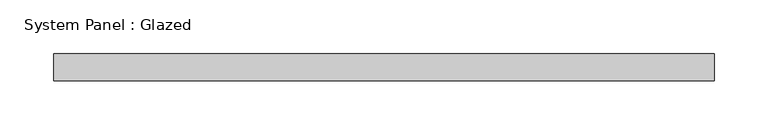
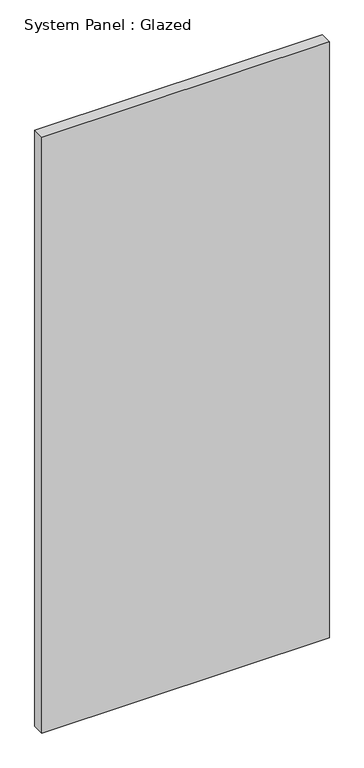
"""IFC4 building model written with IfcOpenShell, lengths in millimetres: plate geometry, System Panel : Glazed."""

from ifc_helpers import new_model, si_unit, origin, origin_with_axes, place, context, project, spatial, polyline, outline, extrude, source, transform, mapped, element, save


def system_panel_glazed_296d4335(model_context):
    return source(origin(), model_context, "Body", "SweptSolid", [
        extrude(outline(polyline([(307.975, 19.05), (-307.975, 19.05), (-307.975, 44.45), (307.975, 44.45), (307.975, 19.05)])), origin_with_axes(), (0.0, 0.0, 1.0), 1348.8013618),
    ])


if __name__ == "__main__":
    model = new_model("IFC4")
    model_context = context("Model", 3, world=origin())
    ifc_project = project(units=[si_unit("LENGTHUNIT", "METRE", prefix="MILLI")], contexts=[model_context])
    site = spatial("IfcSite", under=ifc_project)
    building = spatial("IfcBuilding", under=site)
    placement = place(None, origin())
    system_panel_glazed_shape = system_panel_glazed_296d4335(model_context)
    element("IfcPlate", 1, ObjectType="System Panel : Glazed", at=placement, inside=building, context=model_context, shape_type="MappedRepresentation", body=[
        mapped(system_panel_glazed_shape, transform((0.0, 0.0, 0.0), x_axis=(1.0, 0.0, 0.0), y_axis=(0.0, 1.0, 0.0), z_axis=(0.0, 0.0, 1.0))),
    ])
    save(model, "model.ifc")

# Revit data of these elements
# Type "System Panel : Glazed"
#   Construction Type Id = "GSP4R"
#   Analytic Construction = "1/8 in Pilkington single glazing"
#   Visual Light Transmittance = 0.9
#   Solar Heat Gain Coefficient = 0.86
#   Heat Transfer Coefficient (U) = 1.18115 BTU/(h·ft²·°F)
#   Define Thermal Properties by = 1
# Element 1 (IfcPlate, "System Panel : Glazed")
#   Materials on its faces: "Glass"
# Materials
#   "Glass": class "Glass", colour RGB 0 128 192, transparency 0.75, Description = "Soda Lime Glass", Cost = 0
